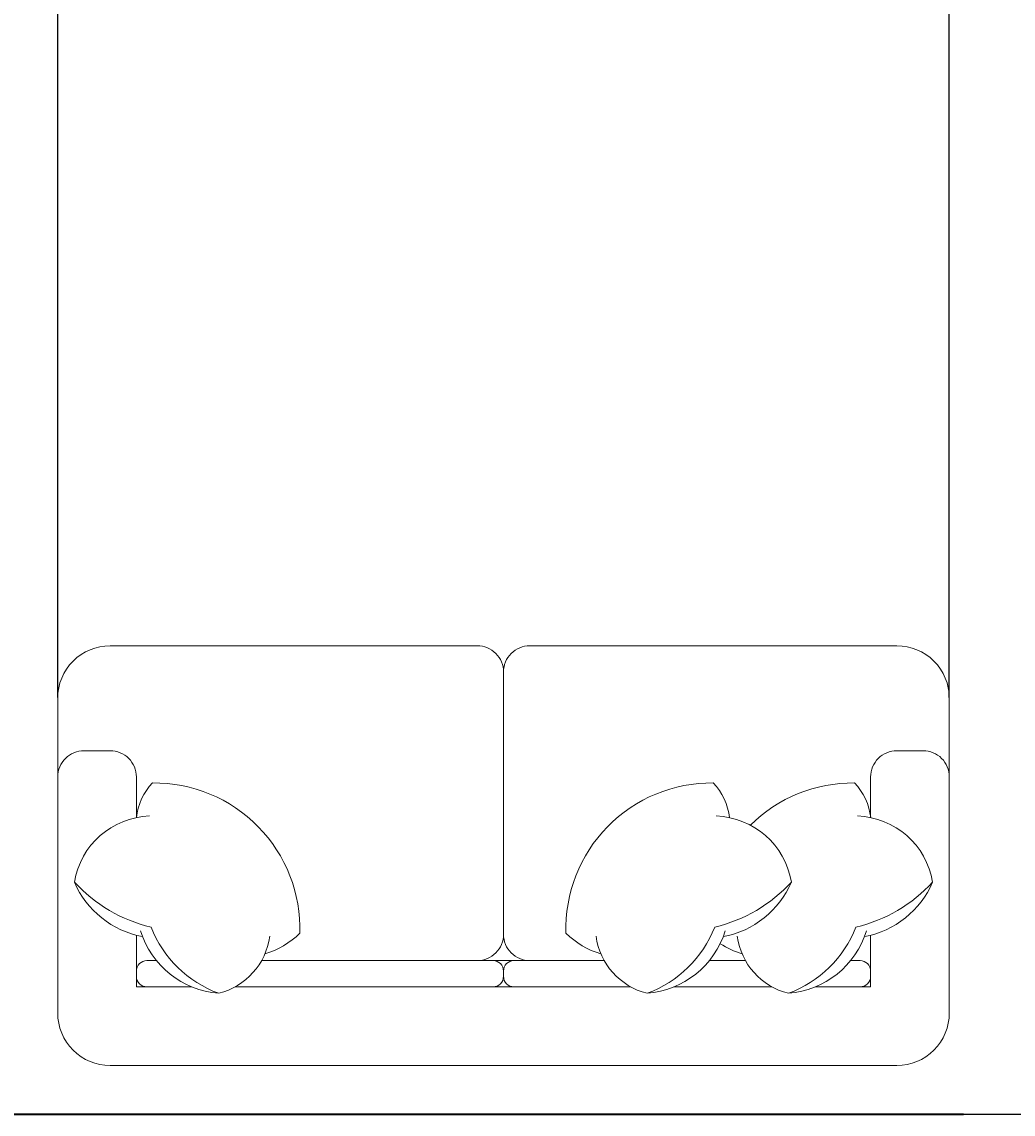
# Model space of a CAD drawing. Units: inches. Extents: x 1088 to 1703, y 668 to 1875.
# Tile 10 of 45: x 1244 to 1314, y 1419 to 1496. Entities that reach past the tile are written whole.
import ezdxf

# ---------------------------------------------------------------- set-up
doc = ezdxf.new("R2010")
doc.units = ezdxf.units.IN
for name, color, linetype, lineweight in [('A-ANNO-DIMS', 2, 'Continuous', 18), ('A-FLOR-EVTR', 5, 'Continuous', 25), ('A-FURN', 8, 'Continuous', 13), ('A-WALL', 7, 'Continuous', 35)]:
    doc.layers.add(name, color=color, linetype=linetype, lineweight=lineweight)
doc.styles.get("Standard").update_dxf_attribs({"font": 'arial.ttf'})
doc.dimstyles.get("Standard").update_dxf_attribs({"dimtxt": 0.18, "dimasz": 0.18, "dimexe": 0.18, "dimexo": 0.0625, "dimgap": 0.09, "dimtad": 0, "dimtih": 1, "dimtoh": 1, "dimdec": 4, "dimzin": 0, "dimdsep": 46, "dimtxsty": 'Standard', "dimcen": 0.09, "dimadec": 0, "dimazin": 0, "dimtfac": 1, "dimtdec": 4, "dimtofl": 0, "dimtmove": 0, "dimatfit": 3, "dimfxl": 1, "dimtolj": 1, "dimtzin": 0, "dimarcsym": 0})

# ---------------------------------------------------------------- blocks, each defined once
blk = doc.blocks.new('*D36')
at = {"layer": 'A-ANNO-DIMS', "color": 0, "lineweight": -2, "transparency": 16777216}
for p, q in [((1246.852, 1448.35), (1246.852, 1857.788)), ((1247.032, 1857.608), (1277.777, 1857.608)), ((1309.172, 1857.608), (1278.427, 1857.608)), ((1309.352, 1448.35), (1309.352, 1857.788))]:
    blk.add_line(p, q, dxfattribs=at)
at = {"layer": 'A-ANNO-DIMS', "color": 0, "transparency": 16777216}
for points in [[(1247.032, 1857.638), (1247.032, 1857.578), (1246.852, 1857.608)], [(1309.172, 1857.638), (1309.172, 1857.578), (1309.352, 1857.608)]]:
    blk.add_solid(points, dxfattribs=at)
at = {"layer": 'Defpoints', "color": 0, "transparency": 16777216}
for p in [(1309.352, 1857.608), (1246.852, 1448.287), (1309.352, 1448.287)]:
    blk.add_point(p, dxfattribs=at)
at = {"layer": 'A-ANNO-DIMS', "color": 0, "transparency": 16777216, "insert": (1278.102, 1857.608), "char_height": 0.18, "attachment_point": 5}
blk.add_mtext('\\A1;62.5', dxfattribs=at)

msp = doc.modelspace()

# ---------------------------------------------------------------- linework, layer by layer
at = {"layer": 'A-FLOR-EVTR'}
msp.add_line((1294.845, 1419.144), (1354.845, 1419.144), dxfattribs=at)
at = {"layer": 'A-FURN', "ltscale": 0.03}
msp.add_lwpolyline([(1276.264, 1451.964, -0.414214), (1278.102, 1450.125, -0.414214), (1279.94, 1451.964), (1305.675, 1451.964, -0.414214), (1309.352, 1448.287), (1309.352, 1426.229, -0.414214), (1305.675, 1422.552), (1250.529, 1422.552, -0.414214), (1246.852, 1426.229), (1246.852, 1448.287, -0.414214), (1250.529, 1451.964), (1276.264, 1451.964, -0.414214), (1278.102, 1450.125, -0.414214), (1279.94, 1451.964)], format="xyb", dxfattribs=at)
at = {"layer": 'A-FURN'}
for points in [[(1276.264, 1429.905, 0.414214), (1278.102, 1431.743), (1278.102, 1450.125, 0.414214)], [(1279.94, 1429.905, -0.414214), (1278.102, 1431.743), (1278.102, 1450.125, -0.414214)], [(1246.852, 1442.773, -0.414214), (1248.691, 1444.611), (1250.529, 1444.611, -0.414214), (1252.367, 1442.773), (1252.367, 1439.925)], [(1303.837, 1439.925), (1303.837, 1442.773, -0.414214), (1305.675, 1444.611), (1307.513, 1444.611, -0.414214), (1309.352, 1442.773)], [(1252.363, 1439.924, -0.165541), (1253.5, 1442.352, -0.425989), (1263.824, 1431.822, -0.121523), (1261.373, 1430.371, 7.115464)], [(1293.939, 1439.924, 0.165541), (1292.801, 1442.352, 0.425989), (1282.478, 1431.822, 0.121523), (1284.928, 1430.371, -7.115464)], [(1303.841, 1439.924, 0.165541), (1302.704, 1442.352, 0.200231), (1295.407, 1439.394, 0.121523)], [(1253.29, 1440.036, 0.356772), (1248.022, 1435.402, 0.249542), (1252.795, 1431.584, -9.61688)], [(1293.012, 1440.036, -0.356772), (1298.279, 1435.402, -0.249542), (1293.507, 1431.584, 9.61688)], [(1302.914, 1440.036, -0.356772), (1308.182, 1435.402, -0.249542), (1303.409, 1431.584, 9.61688)], [(1248.022, 1435.402, 0.14773), (1253.395, 1432.243, 0.213343), (1258.135, 1427.61, 0.178662)], [(1298.279, 1435.402, -0.14773), (1292.907, 1432.243, -0.213343), (1288.166, 1427.61, -0.178662)], [(1308.182, 1435.402, -0.14773), (1302.809, 1432.243, -0.213343), (1298.069, 1427.61, -0.178662)], [(1252.653, 1431.991, 0.306663), (1258.135, 1427.61, 0.30633), (1261.717, 1431.611, -0.872847)], [(1276.264, 1429.905, 0.414214), (1278.102, 1431.743)], [(1279.94, 1429.905, -0.414214), (1278.102, 1431.743)], [(1293.649, 1431.991, -0.306663), (1288.166, 1427.61, -0.30633), (1284.585, 1431.611, 0.872847)], [(1303.551, 1431.991, -0.306663), (1298.069, 1427.61, -0.30633), (1294.487, 1431.611, 0.872847)], [(1299.97, 1428.067), (1303.837, 1428.067), (1303.837, 1431.679, -0.414214)], [(1293.29, 1431.089, 0.071865), (1294.831, 1430.371, -7.115464)], [(1253.77, 1429.905), (1253.102, 1429.905, 0.414214), (1252.367, 1429.17), (1252.367, 1428.802, 0.414214), (1253.102, 1428.067)], [(1259.292, 1428.067), (1277.367, 1428.067, 0.414214), (1278.102, 1428.802), (1278.102, 1429.17, 0.414214), (1277.367, 1429.905), (1261.143, 1429.905, 0.414214)], [(1287.009, 1428.067), (1278.837, 1428.067, -0.414214), (1278.102, 1428.802), (1278.102, 1429.17, -0.414214), (1278.837, 1429.905), (1285.158, 1429.905, -0.414214)], [(1292.532, 1429.905), (1295.061, 1429.905, -0.414214)], [(1302.434, 1429.905), (1303.102, 1429.905, -0.414214), (1303.837, 1429.17), (1303.837, 1428.802, -0.414214), (1303.102, 1428.067)], [(1253.102, 1428.067), (1256.234, 1428.067, 0.414214)], [(1296.912, 1428.067), (1290.068, 1428.067, -0.414214)], [(1303.102, 1428.067), (1299.97, 1428.067, -0.414214)]]:
    msp.add_lwpolyline(points, format="xyb", dxfattribs=at)
for points in [[(1252.367, 1431.679), (1252.367, 1428.067), (1256.234, 1428.067)], [(1259.292, 1428.067), (1287.009, 1428.067)], [(1290.068, 1428.067), (1296.912, 1428.067)]]:
    msp.add_lwpolyline(points, dxfattribs=at)
msp.add_lwpolyline([(1277.367, 1428.067), (1278.837, 1428.067, -0.414214), (1278.102, 1428.802), (1278.102, 1429.17, -0.414214), (1278.837, 1429.905), (1277.367, 1429.905, -0.414214), (1278.102, 1429.17), (1278.102, 1428.802, -0.414214)], format="xyb", close=True, dxfattribs=at)
at = {"layer": 'A-WALL'}
msp.add_line((1174.845, 1419.144), (1310.352, 1419.144), dxfattribs=at)

# ---------------------------------------------------------------- dimensions: what is measured, and where the dimension line sits
at = {"layer": 'A-ANNO-DIMS'}
dim = msp.add_linear_dim(base=(1309.352, 1857.608), p1=(1246.852, 1448.287), p2=(1309.352, 1448.287), dimstyle='Standard', override={"dimdec": 1, "dimlfac": 1, "dimrnd": 0, "dimzin": 0, "dimdsep": 46, "dimlunit": 2}, dxfattribs=at)
dim.commit()
dim.dimension.update_dxf_attribs({"geometry": '*D36', "text_midpoint": (1278.102, 1857.608)})

doc.saveas('drawing.dxf')
